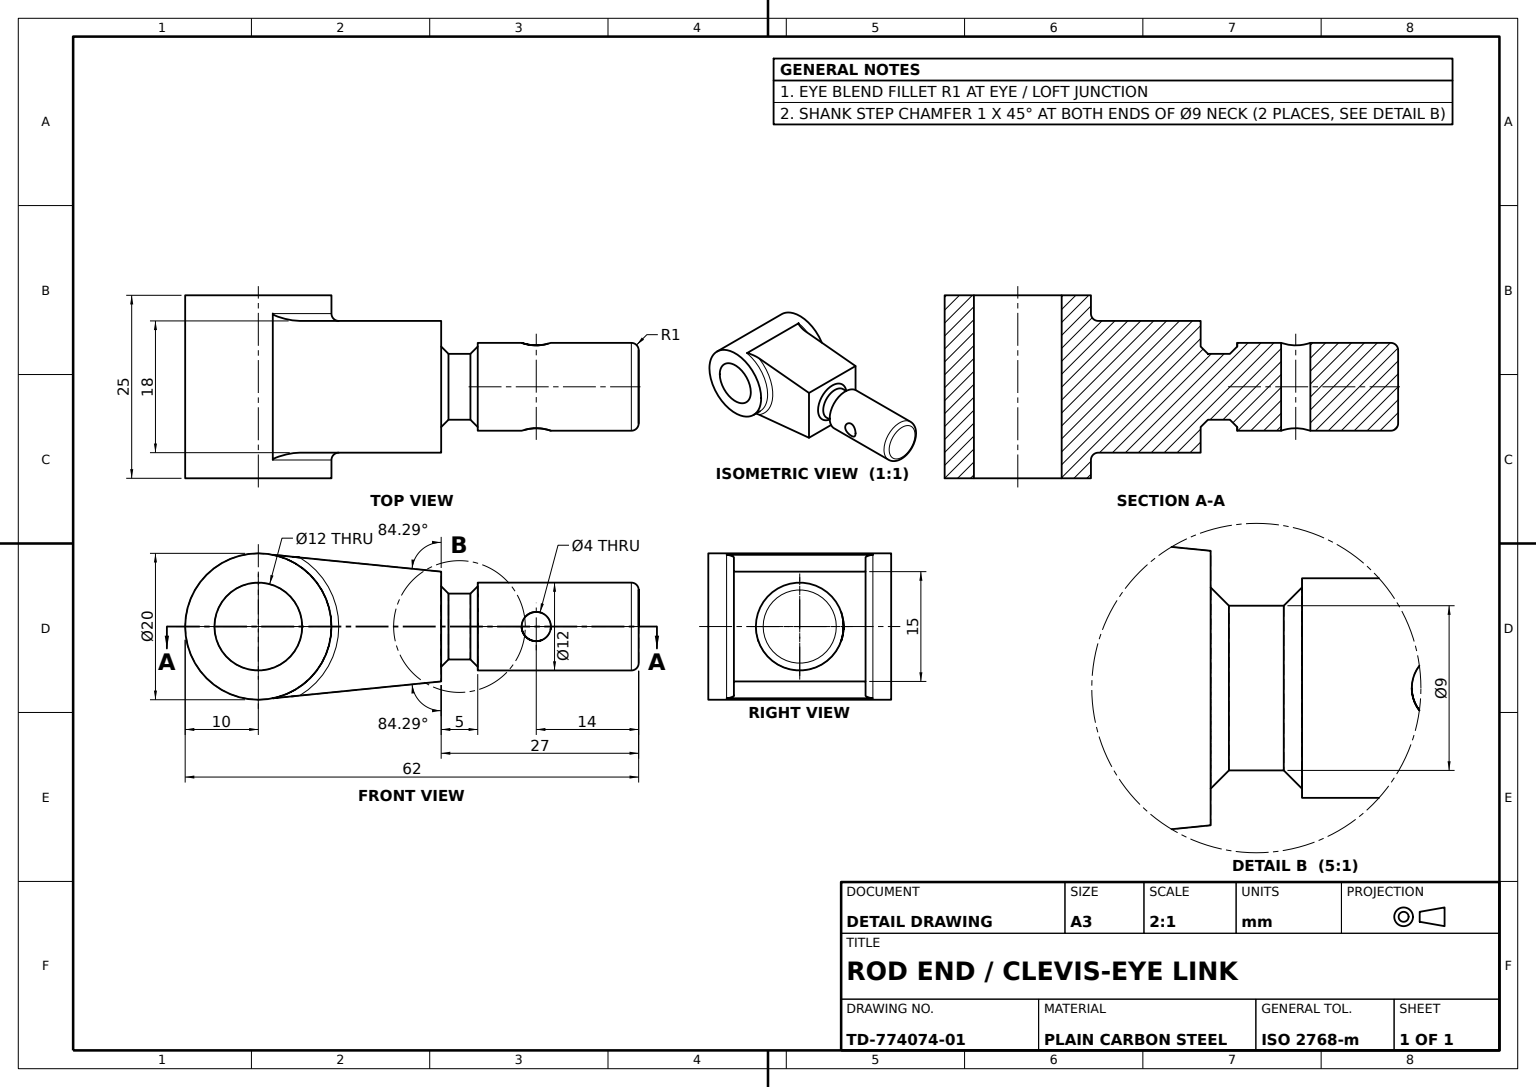
SolidWorks part; units mm, degrees
material "Plain Carbon Steel"
ref_plane "Front Plane" through (0, 0, 0) normal (0, 0, 1) x (1, 0, 0)
ref_plane "Top Plane" through (0, 0, 0) normal (0, 1, 0) x (1, 0, 0)
ref_plane "Right Plane" through (0, 0, 0) normal (1, 0, 0) x (0, 0, -1)
sketch "Shank Profile Ø12" plane through (0, 0, 0) normal (0, 0, 1) x (1, 0, 0)
  circle A0 centre (0, 0) radius 6
  dimension "D1" = 12
extrude "Shank Ø12x27" add sketch "Shank Profile Ø12" along normal blind 27
sketch "Shank Step Profile Ø9" plane through (0, 0, 27) normal (0, 0, 1) x (1, 0, 0)
  circle A0 centre (0, 0) radius 4.5
  circle A1 centre (0, 0) radius 6
  circle A2 centre (0, 0) radius 6
  dimension "D2" = 9
  dimension "D1" = 0
extrude "Shank Step Ø9x5" cut sketch "Shank Step Profile Ø9" against normal blind 5 and the other way through all
sketch "Loft Start Section 18x15" plane through (0, 0, 27) normal (0, 0, 1) x (1, 0, 0)
  line L1 (-9, 7.5) -> (9, 7.5)
  line L2 (-9, 7.5) -> (-9, -7.5)
  line L3 (-9, -7.5) -> (9, -7.5)
  line L4 (9, 7.5) -> (9, -7.5)
  line L5 (-9, 7.5) -> (9, -7.5) construction
  line L6 (-9, -7.5) -> (9, 7.5) construction
  point P0 (0, 0)
  dimension "D1" = 18
  dimension "D2" = 15
ref_plane "Eye Block Plane" through (0, 0, 52) normal (0, 0, 1) x (1, 0, 0)
sketch "Eye Profile Ø20" plane through (0, 0, 0) normal (1, 0, 0) x (0, 0, -1)
  line L0 (-52, 55) -> (-52, -55) construction
  circle A0 centre (-52, 0) radius 10
  circle A1 centre (-52, 0) radius 6
  dimension "D1" = 20
  dimension "D2" = 12
extrude "Eye Boss Ø20x25" add sketch "Eye Profile Ø20" along normal mid plane 25 separate body
sketch "Loft End Section 18x20" plane through (0, 0, 52) normal (0, 0, 1) x (1, 0, 0)
  line L1 (-9, 10) -> (9, 10)
  line L2 (-9, 10) -> (-9, -10)
  line L3 (-9, -10) -> (9, -10)
  line L4 (9, 10) -> (9, -10)
  line L5 (-9, 10) -> (9, -10) construction
  line L6 (-9, -10) -> (9, 10) construction
  point P0 (0, 0)
  dimension "D1" = 18
  dimension "D2" = 20
loft "Shank To Eye Transition" add profiles "Loft End Section 18x20", "Loft Start Section 18x15"
sketch "Eye Bore Profile" plane through (12.5, 0, 0) normal (1, 0, 0) x (0, 0, -1)
  circle A0 centre (-52, 0) radius 6 construction
  circle A1 centre (-52, 0) radius 6
extrude "Eye Bore" cut sketch "Eye Bore Profile" against normal blind 35
sketch "Cross Hole Profile Ø4" plane through (0, 0, 0) normal (1, 0, 0) x (0, 0, -1)
  line L0 (0, -6) -> (0, 6) construction
  circle A0 centre (-14, 0) radius 2
  dimension "D1" = 4
  dimension "D2" = 14
extrude "Cross Hole Ø4" cut sketch "Cross Hole Profile Ø4" against normal through all both and the other way through all
fillet "Eye Blend Fillet R1" radius 1 3 edges at (-9, 0, 42) (9, 0, 42) (6, 0, 0)
chamfer "Shank Step Chamfer 1x45" distance 1 angle 45 2 edges at (4.5, 0, 22)
